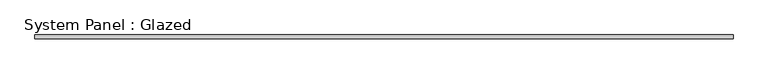
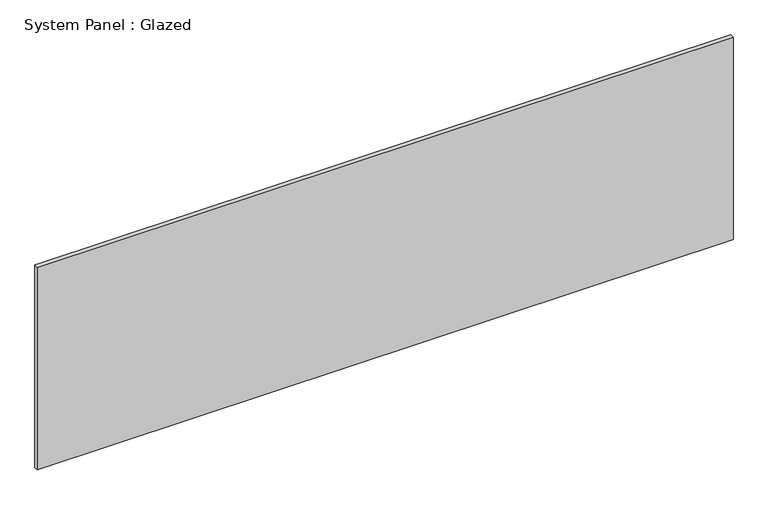
"""IFC4 building model written with IfcOpenShell, lengths in millimetres: plate geometry, System Panel : Glazed."""

from ifc_helpers import new_model, si_unit, origin, origin_with_axes, place, context, project, spatial, polyline, outline, extrude, source, transform, mapped, element, save


def system_panel_glazed_86bade12(model_context):
    return source(origin(), model_context, "Body", "SweptSolid", [
        extrude(outline(polyline([(2371.5343658, 19.05), (-2371.5343658, 19.05), (-2371.5343658, 44.45), (2371.5343658, 44.45), (2371.5343658, 19.05)])), origin_with_axes(), (0.0, 0.0, 1.0), 1460.5),
    ])


if __name__ == "__main__":
    model = new_model("IFC4")
    model_context = context("Model", 3, world=origin())
    ifc_project = project(units=[si_unit("LENGTHUNIT", "METRE", prefix="MILLI")], contexts=[model_context])
    site = spatial("IfcSite", under=ifc_project)
    building = spatial("IfcBuilding", under=site)
    placement = place(None, origin())
    system_panel_glazed_shape = system_panel_glazed_86bade12(model_context)
    element("IfcPlate", 1, ObjectType="System Panel : Glazed", at=placement, inside=building, context=model_context, shape_type="MappedRepresentation", body=[
        mapped(system_panel_glazed_shape, transform((0.0, 0.0, 0.0), x_axis=(1.0, 0.0, 0.0), y_axis=(0.0, 1.0, 0.0), z_axis=(0.0, 0.0, 1.0))),
    ])
    save(model, "model.ifc")

# Revit data of these elements
# Type "System Panel : Glazed"
#   Construction Type Id = "GSP4R"
#   Analytic Construction = "1/8 in Pilkington single glazing"
#   Visual Light Transmittance = 0.9
#   Solar Heat Gain Coefficient = 0.86
#   Heat Transfer Coefficient (U) = 1.18115 BTU/(h·ft²·°F)
# Element 1 (IfcPlate, "System Panel : Glazed")
#   Materials on its faces: "Glass"
# Materials
#   "Glass": class "Glass", colour RGB 0 128 192, transparency 0.75, Description = "Soda Lime Glass", Cost = 0
